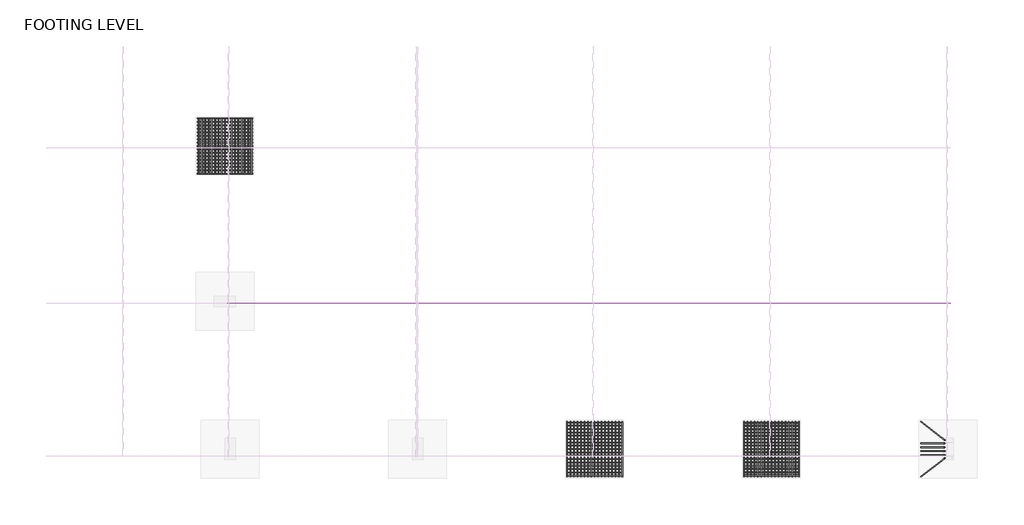
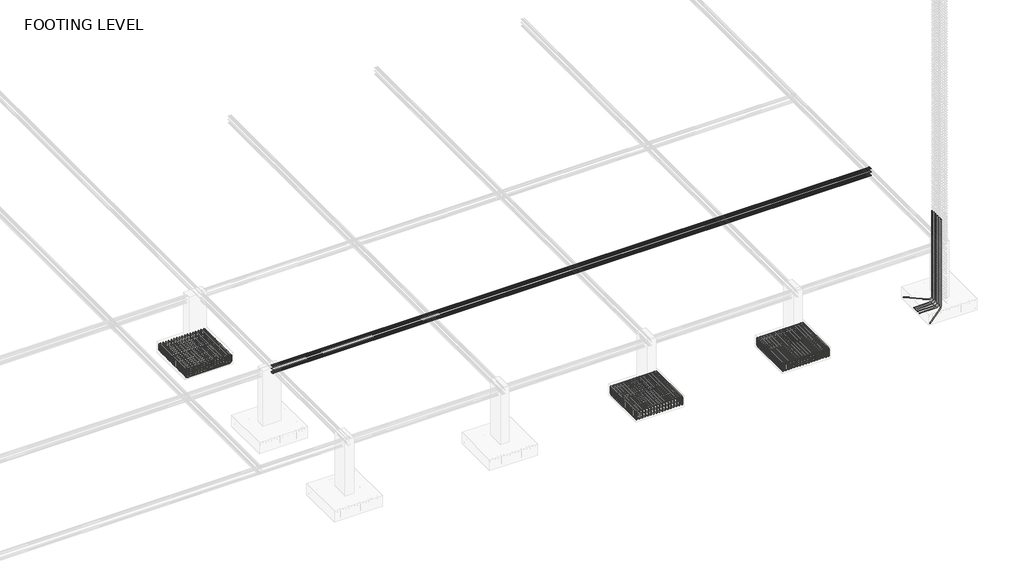
# One storey, part 6 of 19: 16 reinforcing bars.
"""IFC4 building model written with IfcOpenShell, lengths in millimetres."""

from ifc_helpers import new_model, si_unit, point, frame, origin, place, context, project, spatial, polyline, circle_curve, trimmed, segment, composite_curve, source, transform, mapped, element, save
from ifc_brep_helpers import swept_disk

model = new_model("IFC4")

# Units and contexts
model_context = context("Model", 3, world=origin())
ifc_project = project(units=[si_unit("LENGTHUNIT", "METRE", prefix="MILLI")], contexts=[model_context])

# Site, building, storey
site = spatial("IfcSite", under=ifc_project)
building = spatial("IfcBuilding", under=site)
storey = spatial("IfcBuildingStorey", under=building, Name="FOOTING LEVEL", Elevation=-3048.0)

# Reinforcing bars
placement = place(None, origin())
element("IfcReinforcingBar", 1, at=placement, inside=storey, context=model_context, shape_type="SolidModel", body=[
    swept_disk(composite_curve([segment(polyline([(32151.2177574, -27441.3062866, 1300.0821641), (32151.2177574, -27441.3062866, -3426.35)]), True, "CONTINUOUS"), segment(trimmed(circle_curve(frame((32030.1399051, -27346.7099009, -3426.35), z_axis=(0.6156614753255063, 0.7880107536068408, 0.0), x_axis=(121.07785230000081, -94.59638569999879, 0.0)), 153.65), [point((32151.2177574, -27441.3062866, -3426.35))], [point((32030.1399051, -27346.7099009, -3580.0))], True, "CARTESIAN"), True, "CONTINUOUS"), segment(polyline([(32030.1399051, -27346.7099009, -3580.0), (31124.1613605, -26638.881886, -3580.0)]), True, "CONTINUOUS")], self_intersect=False), 16.15),
])
element("IfcReinforcingBar", 2, at=placement, inside=storey, context=model_context, shape_type="SolidModel", body=[
    swept_disk(composite_curve([segment(polyline([(32151.8797141, -28220.6474683, 1296.5097943), (32151.8797141, -28220.6474683, -3426.35)]), True, "CONTINUOUS"), segment(trimmed(circle_curve(frame((32030.8018618, -28315.243854, -3426.35), z_axis=(-0.6156614753255063, 0.7880107536068408, 0.0), x_axis=(121.07785230000081, 94.59638569999879, 0.0)), 153.65), [point((32151.8797141, -28220.6474683, -3426.35))], [point((32030.8018618, -28315.243854, -3580.0))], True, "CARTESIAN"), True, "CONTINUOUS"), segment(polyline([(32030.8018618, -28315.243854, -3580.0), (31127.9113605, -29020.6592249, -3580.0)]), True, "CONTINUOUS")], self_intersect=False), 16.15),
])
reinforcing_bar_shape = source(origin(), model_context, "Body", "SolidModel", [
    swept_disk(composite_curve([segment(polyline([(32149.6087563, -28081.7876394, 1313.4672881), (32149.6087563, -28081.7876394, -3426.35)]), True, "CONTINUOUS"), segment(trimmed(circle_curve(frame((31995.9587563, -28081.7876394, -3426.35), z_axis=(0.0, 1.0, 0.0), x_axis=(153.65000000000146, 0.0, 0.0)), 153.65), [point((32149.6087563, -28081.7876394, -3426.35))], [point((31995.9587563, -28081.7876394, -3580.0))], True, "CARTESIAN"), True, "CONTINUOUS"), segment(polyline([(31995.9587563, -28081.7876394, -3580.0), (31112.5587563, -28081.7876394, -3580.0)]), True, "CONTINUOUS")], self_intersect=False), 16.15),
])
element("IfcReinforcingBar", 3, at=placement, inside=storey, context=model_context, shape_type="MappedRepresentation", body=[
    mapped(reinforcing_bar_shape, transform((0.0, 0.0, 0.0), x_axis=(1.0, 0.0, 0.0), y_axis=(0.0, 1.0, 0.0), z_axis=(0.0, 0.0, 1.0))),
    mapped(reinforcing_bar_shape, transform((0.0, 165.6818922, 0.0), x_axis=(1.0, 0.0, 0.0), y_axis=(0.0, 1.0, 0.0), z_axis=(0.0, 0.0, 1.0))),
    mapped(reinforcing_bar_shape, transform((0.0, 331.3637844, 0.0), x_axis=(1.0, 0.0, 0.0), y_axis=(0.0, 1.0, 0.0), z_axis=(0.0, 0.0, 1.0))),
    mapped(reinforcing_bar_shape, transform((0.0, 497.0456766, 0.0), x_axis=(1.0, 0.0, 0.0), y_axis=(0.0, 1.0, 0.0), z_axis=(0.0, 0.0, 1.0))),
])
reinforcing_bar_2_shape = source(origin(), model_context, "Body", "SolidModel", [
    swept_disk(composite_curve([segment(polyline([(25879.8587563, -28952.7516566, -3148.0), (25879.8587563, -28952.7516566, -3470.1)]), True, "CONTINUOUS"), segment(trimmed(circle_curve(frame((25789.6587563, -28952.7516566, -3470.1), z_axis=(0.0, 1.0, 0.0), x_axis=(90.20000000000073, 0.0, 0.0)), 90.2), [point((25879.8587563, -28952.7516566, -3470.1))], [point((25789.6587563, -28952.7516566, -3560.3))], True, "CARTESIAN"), True, "CONTINUOUS"), segment(polyline([(25789.6587563, -28952.7516566, -3560.3), (23595.4587563, -28952.7516566, -3560.3)]), True, "CONTINUOUS"), segment(trimmed(circle_curve(frame((23595.4587563, -28952.7516566, -3470.1), z_axis=(0.0, 1.0, 0.0), x_axis=(0.0, 0.0, -90.20000000000027)), 90.2), [point((23595.4587563, -28952.7516566, -3560.3))], [point((23505.2587563, -28952.7516566, -3470.1))], True, "CARTESIAN"), True, "CONTINUOUS"), segment(polyline([(23505.2587563, -28952.7516566, -3470.1), (23505.2587563, -28952.7516566, -3148.0)]), True, "CONTINUOUS")], self_intersect=False), 12.7),
])
element("IfcReinforcingBar", 4, at=placement, inside=storey, context=model_context, shape_type="MappedRepresentation", body=[
    mapped(reinforcing_bar_2_shape, transform((0.0, 0.0, 0.0), x_axis=(1.0, 0.0, 0.0), y_axis=(0.0, 1.0, 0.0), z_axis=(0.0, 0.0, 1.0))),
    mapped(reinforcing_bar_2_shape, transform((0.0, 140.8090411, 0.0), x_axis=(1.0, 0.0, 0.0), y_axis=(0.0, 1.0, 0.0), z_axis=(0.0, 0.0, 1.0))),
    mapped(reinforcing_bar_2_shape, transform((0.0, 281.6180821, 0.0), x_axis=(1.0, 0.0, 0.0), y_axis=(0.0, 1.0, 0.0), z_axis=(0.0, 0.0, 1.0))),
    mapped(reinforcing_bar_2_shape, transform((0.0, 422.4271232, 0.0), x_axis=(1.0, 0.0, 0.0), y_axis=(0.0, 1.0, 0.0), z_axis=(0.0, 0.0, 1.0))),
    mapped(reinforcing_bar_2_shape, transform((0.0, 563.2361643, 0.0), x_axis=(1.0, 0.0, 0.0), y_axis=(0.0, 1.0, 0.0), z_axis=(0.0, 0.0, 1.0))),
    mapped(reinforcing_bar_2_shape, transform((0.0, 704.0452054, 0.0), x_axis=(1.0, 0.0, 0.0), y_axis=(0.0, 1.0, 0.0), z_axis=(0.0, 0.0, 1.0))),
    mapped(reinforcing_bar_2_shape, transform((0.0, 844.8542464, 0.0), x_axis=(1.0, 0.0, 0.0), y_axis=(0.0, 1.0, 0.0), z_axis=(0.0, 0.0, 1.0))),
    mapped(reinforcing_bar_2_shape, transform((0.0, 985.6632875, 0.0), x_axis=(1.0, 0.0, 0.0), y_axis=(0.0, 1.0, 0.0), z_axis=(0.0, 0.0, 1.0))),
    mapped(reinforcing_bar_2_shape, transform((0.0, 1126.4723286, 0.0), x_axis=(1.0, 0.0, 0.0), y_axis=(0.0, 1.0, 0.0), z_axis=(0.0, 0.0, 1.0))),
    mapped(reinforcing_bar_2_shape, transform((0.0, 1267.2813697, 0.0), x_axis=(1.0, 0.0, 0.0), y_axis=(0.0, 1.0, 0.0), z_axis=(0.0, 0.0, 1.0))),
    mapped(reinforcing_bar_2_shape, transform((0.0, 1408.0904107, 0.0), x_axis=(1.0, 0.0, 0.0), y_axis=(0.0, 1.0, 0.0), z_axis=(0.0, 0.0, 1.0))),
    mapped(reinforcing_bar_2_shape, transform((0.0, 1548.8994518, 0.0), x_axis=(1.0, 0.0, 0.0), y_axis=(0.0, 1.0, 0.0), z_axis=(0.0, 0.0, 1.0))),
    mapped(reinforcing_bar_2_shape, transform((0.0, 1689.7084929, 0.0), x_axis=(1.0, 0.0, 0.0), y_axis=(0.0, 1.0, 0.0), z_axis=(0.0, 0.0, 1.0))),
    mapped(reinforcing_bar_2_shape, transform((0.0, 1830.517534, 0.0), x_axis=(1.0, 0.0, 0.0), y_axis=(0.0, 1.0, 0.0), z_axis=(0.0, 0.0, 1.0))),
    mapped(reinforcing_bar_2_shape, transform((0.0, 1971.326575, 0.0), x_axis=(1.0, 0.0, 0.0), y_axis=(0.0, 1.0, 0.0), z_axis=(0.0, 0.0, 1.0))),
    mapped(reinforcing_bar_2_shape, transform((0.0, 2112.1356161, 0.0), x_axis=(1.0, 0.0, 0.0), y_axis=(0.0, 1.0, 0.0), z_axis=(0.0, 0.0, 1.0))),
    mapped(reinforcing_bar_2_shape, transform((0.0, 2252.9446572, 0.0), x_axis=(1.0, 0.0, 0.0), y_axis=(0.0, 1.0, 0.0), z_axis=(0.0, 0.0, 1.0))),
])
reinforcing_bar_3_shape = source(origin(), model_context, "Body", "SolidModel", [
    swept_disk(composite_curve([segment(polyline([(25879.8587563, -26677.3596072, -3548.0), (25879.8587563, -26677.3596072, -3225.9)]), True, "CONTINUOUS"), segment(trimmed(circle_curve(frame((25789.6587563, -26677.3596072, -3225.9), z_axis=(0.0, -1.0, 0.0), x_axis=(90.20000000000073, 0.0, 0.0)), 90.2), [point((25879.8587563, -26677.3596072, -3225.9))], [point((25789.6587563, -26677.3596072, -3135.7))], True, "CARTESIAN"), True, "CONTINUOUS"), segment(polyline([(25789.6587563, -26677.3596072, -3135.7), (23595.4587563, -26677.3596072, -3135.7)]), True, "CONTINUOUS"), segment(trimmed(circle_curve(frame((23595.4587563, -26677.3596072, -3225.9), z_axis=(0.0, -1.0, 0.0), x_axis=(0.0, 0.0, 90.20000000000027)), 90.2), [point((23595.4587563, -26677.3596072, -3135.7))], [point((23505.2587563, -26677.3596072, -3225.9))], True, "CARTESIAN"), True, "CONTINUOUS"), segment(polyline([(23505.2587563, -26677.3596072, -3225.9), (23505.2587563, -26677.3596072, -3548.0)]), True, "CONTINUOUS")], self_intersect=False), 12.7),
])
element("IfcReinforcingBar", 5, at=placement, inside=storey, context=model_context, shape_type="MappedRepresentation", body=[
    mapped(reinforcing_bar_3_shape, transform((0.0, 0.0, 0.0), x_axis=(1.0, 0.0, 0.0), y_axis=(0.0, 1.0, 0.0), z_axis=(0.0, 0.0, 1.0))),
    mapped(reinforcing_bar_3_shape, transform((0.0, -143.8496077, 0.0), x_axis=(1.0, 0.0, 0.0), y_axis=(0.0, 1.0, 0.0), z_axis=(0.0, 0.0, 1.0))),
    mapped(reinforcing_bar_3_shape, transform((0.0, -287.6992155, 0.0), x_axis=(1.0, 0.0, 0.0), y_axis=(0.0, 1.0, 0.0), z_axis=(0.0, 0.0, 1.0))),
    mapped(reinforcing_bar_3_shape, transform((0.0, -431.5488232, 0.0), x_axis=(1.0, 0.0, 0.0), y_axis=(0.0, 1.0, 0.0), z_axis=(0.0, 0.0, 1.0))),
    mapped(reinforcing_bar_3_shape, transform((0.0, -575.398431, 0.0), x_axis=(1.0, 0.0, 0.0), y_axis=(0.0, 1.0, 0.0), z_axis=(0.0, 0.0, 1.0))),
    mapped(reinforcing_bar_3_shape, transform((0.0, -719.2480387, 0.0), x_axis=(1.0, 0.0, 0.0), y_axis=(0.0, 1.0, 0.0), z_axis=(0.0, 0.0, 1.0))),
    mapped(reinforcing_bar_3_shape, transform((0.0, -863.0976465, 0.0), x_axis=(1.0, 0.0, 0.0), y_axis=(0.0, 1.0, 0.0), z_axis=(0.0, 0.0, 1.0))),
    mapped(reinforcing_bar_3_shape, transform((0.0, -1006.9472542, 0.0), x_axis=(1.0, 0.0, 0.0), y_axis=(0.0, 1.0, 0.0), z_axis=(0.0, 0.0, 1.0))),
    mapped(reinforcing_bar_3_shape, transform((0.0, -1150.796862, 0.0), x_axis=(1.0, 0.0, 0.0), y_axis=(0.0, 1.0, 0.0), z_axis=(0.0, 0.0, 1.0))),
    mapped(reinforcing_bar_3_shape, transform((0.0, -1294.6464697, 0.0), x_axis=(1.0, 0.0, 0.0), y_axis=(0.0, 1.0, 0.0), z_axis=(0.0, 0.0, 1.0))),
    mapped(reinforcing_bar_3_shape, transform((0.0, -1438.4960775, 0.0), x_axis=(1.0, 0.0, 0.0), y_axis=(0.0, 1.0, 0.0), z_axis=(0.0, 0.0, 1.0))),
    mapped(reinforcing_bar_3_shape, transform((0.0, -1582.3456852, 0.0), x_axis=(1.0, 0.0, 0.0), y_axis=(0.0, 1.0, 0.0), z_axis=(0.0, 0.0, 1.0))),
    mapped(reinforcing_bar_3_shape, transform((0.0, -1726.195293, 0.0), x_axis=(1.0, 0.0, 0.0), y_axis=(0.0, 1.0, 0.0), z_axis=(0.0, 0.0, 1.0))),
    mapped(reinforcing_bar_3_shape, transform((0.0, -1870.0449007, 0.0), x_axis=(1.0, 0.0, 0.0), y_axis=(0.0, 1.0, 0.0), z_axis=(0.0, 0.0, 1.0))),
    mapped(reinforcing_bar_3_shape, transform((0.0, -2013.8945085, 0.0), x_axis=(1.0, 0.0, 0.0), y_axis=(0.0, 1.0, 0.0), z_axis=(0.0, 0.0, 1.0))),
    mapped(reinforcing_bar_3_shape, transform((0.0, -2157.7441162, 0.0), x_axis=(1.0, 0.0, 0.0), y_axis=(0.0, 1.0, 0.0), z_axis=(0.0, 0.0, 1.0))),
    mapped(reinforcing_bar_3_shape, transform((0.0, -2301.5937239, 0.0), x_axis=(1.0, 0.0, 0.0), y_axis=(0.0, 1.0, 0.0), z_axis=(0.0, 0.0, 1.0))),
])
reinforcing_bar_4_shape = source(origin(), model_context, "Body", "SolidModel", [
    swept_disk(composite_curve([segment(polyline([(23505.2587563, -29018.3205555, -3173.0), (23505.2587563, -29018.3205555, -3495.1)]), True, "CONTINUOUS"), segment(trimmed(circle_curve(frame((23505.2587563, -28928.1205555, -3495.1), z_axis=(1.0, 0.0, 0.0), x_axis=(0.0, -90.19999999999709, 0.0)), 90.2), [point((23505.2587563, -29018.3205555, -3495.1))], [point((23505.2587563, -28928.1205555, -3585.3))], True, "CARTESIAN"), True, "CONTINUOUS"), segment(polyline([(23505.2587563, -28928.1205555, -3585.3), (23505.2587563, -26733.9205555, -3585.3)]), True, "CONTINUOUS"), segment(trimmed(circle_curve(frame((23505.2587563, -26733.9205555, -3495.1), z_axis=(1.0, 0.0, 0.0), x_axis=(0.0, 0.0, -90.20000000000027)), 90.2), [point((23505.2587563, -26733.9205555, -3585.3))], [point((23505.2587563, -26643.7205555, -3495.1))], True, "CARTESIAN"), True, "CONTINUOUS"), segment(polyline([(23505.2587563, -26643.7205555, -3495.1), (23505.2587563, -26643.7205555, -3173.0)]), True, "CONTINUOUS")], self_intersect=False), 12.7),
])
element("IfcReinforcingBar", 6, at=placement, inside=storey, context=model_context, shape_type="MappedRepresentation", body=[
    mapped(reinforcing_bar_4_shape, transform((0.0, 0.0, 0.0), x_axis=(1.0, 0.0, 0.0), y_axis=(0.0, 1.0, 0.0), z_axis=(0.0, 0.0, 1.0))),
    mapped(reinforcing_bar_4_shape, transform((148.4125, 0.0, 0.0), x_axis=(1.0, 0.0, 0.0), y_axis=(0.0, 1.0, 0.0), z_axis=(0.0, 0.0, 1.0))),
    mapped(reinforcing_bar_4_shape, transform((296.825, 0.0, 0.0), x_axis=(1.0, 0.0, 0.0), y_axis=(0.0, 1.0, 0.0), z_axis=(0.0, 0.0, 1.0))),
    mapped(reinforcing_bar_4_shape, transform((445.2375, 0.0, 0.0), x_axis=(1.0, 0.0, 0.0), y_axis=(0.0, 1.0, 0.0), z_axis=(0.0, 0.0, 1.0))),
    mapped(reinforcing_bar_4_shape, transform((593.65, 0.0, 0.0), x_axis=(1.0, 0.0, 0.0), y_axis=(0.0, 1.0, 0.0), z_axis=(0.0, 0.0, 1.0))),
    mapped(reinforcing_bar_4_shape, transform((742.0625, 0.0, 0.0), x_axis=(1.0, 0.0, 0.0), y_axis=(0.0, 1.0, 0.0), z_axis=(0.0, 0.0, 1.0))),
    mapped(reinforcing_bar_4_shape, transform((890.475, 0.0, 0.0), x_axis=(1.0, 0.0, 0.0), y_axis=(0.0, 1.0, 0.0), z_axis=(0.0, 0.0, 1.0))),
    mapped(reinforcing_bar_4_shape, transform((1038.8875, 0.0, 0.0), x_axis=(1.0, 0.0, 0.0), y_axis=(0.0, 1.0, 0.0), z_axis=(0.0, 0.0, 1.0))),
    mapped(reinforcing_bar_4_shape, transform((1187.3, 0.0, 0.0), x_axis=(1.0, 0.0, 0.0), y_axis=(0.0, 1.0, 0.0), z_axis=(0.0, 0.0, 1.0))),
    mapped(reinforcing_bar_4_shape, transform((1335.7125, 0.0, 0.0), x_axis=(1.0, 0.0, 0.0), y_axis=(0.0, 1.0, 0.0), z_axis=(0.0, 0.0, 1.0))),
    mapped(reinforcing_bar_4_shape, transform((1484.125, 0.0, 0.0), x_axis=(1.0, 0.0, 0.0), y_axis=(0.0, 1.0, 0.0), z_axis=(0.0, 0.0, 1.0))),
    mapped(reinforcing_bar_4_shape, transform((1632.5375, 0.0, 0.0), x_axis=(1.0, 0.0, 0.0), y_axis=(0.0, 1.0, 0.0), z_axis=(0.0, 0.0, 1.0))),
    mapped(reinforcing_bar_4_shape, transform((1780.95, 0.0, 0.0), x_axis=(1.0, 0.0, 0.0), y_axis=(0.0, 1.0, 0.0), z_axis=(0.0, 0.0, 1.0))),
    mapped(reinforcing_bar_4_shape, transform((1929.3625, 0.0, 0.0), x_axis=(1.0, 0.0, 0.0), y_axis=(0.0, 1.0, 0.0), z_axis=(0.0, 0.0, 1.0))),
    mapped(reinforcing_bar_4_shape, transform((2077.775, 0.0, 0.0), x_axis=(1.0, 0.0, 0.0), y_axis=(0.0, 1.0, 0.0), z_axis=(0.0, 0.0, 1.0))),
    mapped(reinforcing_bar_4_shape, transform((2226.1875, 0.0, 0.0), x_axis=(1.0, 0.0, 0.0), y_axis=(0.0, 1.0, 0.0), z_axis=(0.0, 0.0, 1.0))),
    mapped(reinforcing_bar_4_shape, transform((2374.6, 0.0, 0.0), x_axis=(1.0, 0.0, 0.0), y_axis=(0.0, 1.0, 0.0), z_axis=(0.0, 0.0, 1.0))),
])
reinforcing_bar_5_shape = source(origin(), model_context, "Body", "SolidModel", [
    swept_disk(composite_curve([segment(polyline([(23505.2587563, -26643.7205555, -3523.0), (23505.2587563, -26643.7205555, -3200.9)]), True, "CONTINUOUS"), segment(trimmed(circle_curve(frame((23505.2587563, -26733.9205555, -3200.9), z_axis=(1.0, 0.0, 0.0), x_axis=(0.0, 90.20000000000073, 0.0)), 90.2), [point((23505.2587563, -26643.7205555, -3200.9))], [point((23505.2587563, -26733.9205555, -3110.7))], True, "CARTESIAN"), True, "CONTINUOUS"), segment(polyline([(23505.2587563, -26733.9205555, -3110.7), (23505.2587563, -28928.1205555, -3110.7)]), True, "CONTINUOUS"), segment(trimmed(circle_curve(frame((23505.2587563, -28928.1205555, -3200.9), z_axis=(1.0, 0.0, 0.0), x_axis=(0.0, 0.0, 90.20000000000027)), 90.2), [point((23505.2587563, -28928.1205555, -3110.7))], [point((23505.2587563, -29018.3205555, -3200.9))], True, "CARTESIAN"), True, "CONTINUOUS"), segment(polyline([(23505.2587563, -29018.3205555, -3200.9), (23505.2587563, -29018.3205555, -3523.0)]), True, "CONTINUOUS")], self_intersect=False), 12.7),
])
element("IfcReinforcingBar", 7, at=placement, inside=storey, context=model_context, shape_type="MappedRepresentation", body=[
    mapped(reinforcing_bar_5_shape, transform((0.0, 0.0, 0.0), x_axis=(1.0, 0.0, 0.0), y_axis=(0.0, 1.0, 0.0), z_axis=(0.0, 0.0, 1.0))),
    mapped(reinforcing_bar_5_shape, transform((148.4125, 0.0, 0.0), x_axis=(1.0, 0.0, 0.0), y_axis=(0.0, 1.0, 0.0), z_axis=(0.0, 0.0, 1.0))),
    mapped(reinforcing_bar_5_shape, transform((296.825, 0.0, 0.0), x_axis=(1.0, 0.0, 0.0), y_axis=(0.0, 1.0, 0.0), z_axis=(0.0, 0.0, 1.0))),
    mapped(reinforcing_bar_5_shape, transform((445.2375, 0.0, 0.0), x_axis=(1.0, 0.0, 0.0), y_axis=(0.0, 1.0, 0.0), z_axis=(0.0, 0.0, 1.0))),
    mapped(reinforcing_bar_5_shape, transform((593.65, 0.0, 0.0), x_axis=(1.0, 0.0, 0.0), y_axis=(0.0, 1.0, 0.0), z_axis=(0.0, 0.0, 1.0))),
    mapped(reinforcing_bar_5_shape, transform((742.0625, 0.0, 0.0), x_axis=(1.0, 0.0, 0.0), y_axis=(0.0, 1.0, 0.0), z_axis=(0.0, 0.0, 1.0))),
    mapped(reinforcing_bar_5_shape, transform((890.475, 0.0, 0.0), x_axis=(1.0, 0.0, 0.0), y_axis=(0.0, 1.0, 0.0), z_axis=(0.0, 0.0, 1.0))),
    mapped(reinforcing_bar_5_shape, transform((1038.8875, 0.0, 0.0), x_axis=(1.0, 0.0, 0.0), y_axis=(0.0, 1.0, 0.0), z_axis=(0.0, 0.0, 1.0))),
    mapped(reinforcing_bar_5_shape, transform((1187.3, 0.0, 0.0), x_axis=(1.0, 0.0, 0.0), y_axis=(0.0, 1.0, 0.0), z_axis=(0.0, 0.0, 1.0))),
    mapped(reinforcing_bar_5_shape, transform((1335.7125, 0.0, 0.0), x_axis=(1.0, 0.0, 0.0), y_axis=(0.0, 1.0, 0.0), z_axis=(0.0, 0.0, 1.0))),
    mapped(reinforcing_bar_5_shape, transform((1484.125, 0.0, 0.0), x_axis=(1.0, 0.0, 0.0), y_axis=(0.0, 1.0, 0.0), z_axis=(0.0, 0.0, 1.0))),
    mapped(reinforcing_bar_5_shape, transform((1632.5375, 0.0, 0.0), x_axis=(1.0, 0.0, 0.0), y_axis=(0.0, 1.0, 0.0), z_axis=(0.0, 0.0, 1.0))),
    mapped(reinforcing_bar_5_shape, transform((1780.95, 0.0, 0.0), x_axis=(1.0, 0.0, 0.0), y_axis=(0.0, 1.0, 0.0), z_axis=(0.0, 0.0, 1.0))),
    mapped(reinforcing_bar_5_shape, transform((1929.3625, 0.0, 0.0), x_axis=(1.0, 0.0, 0.0), y_axis=(0.0, 1.0, 0.0), z_axis=(0.0, 0.0, 1.0))),
    mapped(reinforcing_bar_5_shape, transform((2077.775, 0.0, 0.0), x_axis=(1.0, 0.0, 0.0), y_axis=(0.0, 1.0, 0.0), z_axis=(0.0, 0.0, 1.0))),
    mapped(reinforcing_bar_5_shape, transform((2226.1875, 0.0, 0.0), x_axis=(1.0, 0.0, 0.0), y_axis=(0.0, 1.0, 0.0), z_axis=(0.0, 0.0, 1.0))),
    mapped(reinforcing_bar_5_shape, transform((2374.6, 0.0, 0.0), x_axis=(1.0, 0.0, 0.0), y_axis=(0.0, 1.0, 0.0), z_axis=(0.0, 0.0, 1.0))),
])
reinforcing_bar_6_shape = source(origin(), model_context, "Body", "SolidModel", [
    swept_disk(composite_curve([segment(polyline([(18259.8587563, -26677.3596072, -3548.0), (18259.8587563, -26677.3596072, -3225.9)]), True, "CONTINUOUS"), segment(trimmed(circle_curve(frame((18169.6587563, -26677.3596072, -3225.9), z_axis=(0.0, -1.0, 0.0), x_axis=(90.20000000000073, 0.0, 0.0)), 90.2), [point((18259.8587563, -26677.3596072, -3225.9))], [point((18169.6587563, -26677.3596072, -3135.7))], True, "CARTESIAN"), True, "CONTINUOUS"), segment(polyline([(18169.6587563, -26677.3596072, -3135.7), (15975.4587563, -26677.3596072, -3135.7)]), True, "CONTINUOUS"), segment(trimmed(circle_curve(frame((15975.4587563, -26677.3596072, -3225.9), z_axis=(0.0, -1.0, 0.0), x_axis=(0.0, 0.0, 90.20000000000027)), 90.2), [point((15975.4587563, -26677.3596072, -3135.7))], [point((15885.2587563, -26677.3596072, -3225.9))], True, "CARTESIAN"), True, "CONTINUOUS"), segment(polyline([(15885.2587563, -26677.3596072, -3225.9), (15885.2587563, -26677.3596072, -3548.0)]), True, "CONTINUOUS")], self_intersect=False), 12.7),
])
element("IfcReinforcingBar", 8, at=placement, inside=storey, context=model_context, shape_type="MappedRepresentation", body=[
    mapped(reinforcing_bar_6_shape, transform((0.0, 0.0, 0.0), x_axis=(1.0, 0.0, 0.0), y_axis=(0.0, 1.0, 0.0), z_axis=(0.0, 0.0, 1.0))),
    mapped(reinforcing_bar_6_shape, transform((0.0, -143.8496077, 0.0), x_axis=(1.0, 0.0, 0.0), y_axis=(0.0, 1.0, 0.0), z_axis=(0.0, 0.0, 1.0))),
    mapped(reinforcing_bar_6_shape, transform((0.0, -287.6992155, 0.0), x_axis=(1.0, 0.0, 0.0), y_axis=(0.0, 1.0, 0.0), z_axis=(0.0, 0.0, 1.0))),
    mapped(reinforcing_bar_6_shape, transform((0.0, -431.5488232, 0.0), x_axis=(1.0, 0.0, 0.0), y_axis=(0.0, 1.0, 0.0), z_axis=(0.0, 0.0, 1.0))),
    mapped(reinforcing_bar_6_shape, transform((0.0, -575.398431, 0.0), x_axis=(1.0, 0.0, 0.0), y_axis=(0.0, 1.0, 0.0), z_axis=(0.0, 0.0, 1.0))),
    mapped(reinforcing_bar_6_shape, transform((0.0, -719.2480387, 0.0), x_axis=(1.0, 0.0, 0.0), y_axis=(0.0, 1.0, 0.0), z_axis=(0.0, 0.0, 1.0))),
    mapped(reinforcing_bar_6_shape, transform((0.0, -863.0976465, 0.0), x_axis=(1.0, 0.0, 0.0), y_axis=(0.0, 1.0, 0.0), z_axis=(0.0, 0.0, 1.0))),
    mapped(reinforcing_bar_6_shape, transform((0.0, -1006.9472542, 0.0), x_axis=(1.0, 0.0, 0.0), y_axis=(0.0, 1.0, 0.0), z_axis=(0.0, 0.0, 1.0))),
    mapped(reinforcing_bar_6_shape, transform((0.0, -1150.796862, 0.0), x_axis=(1.0, 0.0, 0.0), y_axis=(0.0, 1.0, 0.0), z_axis=(0.0, 0.0, 1.0))),
    mapped(reinforcing_bar_6_shape, transform((0.0, -1294.6464697, 0.0), x_axis=(1.0, 0.0, 0.0), y_axis=(0.0, 1.0, 0.0), z_axis=(0.0, 0.0, 1.0))),
    mapped(reinforcing_bar_6_shape, transform((0.0, -1438.4960775, 0.0), x_axis=(1.0, 0.0, 0.0), y_axis=(0.0, 1.0, 0.0), z_axis=(0.0, 0.0, 1.0))),
    mapped(reinforcing_bar_6_shape, transform((0.0, -1582.3456852, 0.0), x_axis=(1.0, 0.0, 0.0), y_axis=(0.0, 1.0, 0.0), z_axis=(0.0, 0.0, 1.0))),
    mapped(reinforcing_bar_6_shape, transform((0.0, -1726.195293, 0.0), x_axis=(1.0, 0.0, 0.0), y_axis=(0.0, 1.0, 0.0), z_axis=(0.0, 0.0, 1.0))),
    mapped(reinforcing_bar_6_shape, transform((0.0, -1870.0449007, 0.0), x_axis=(1.0, 0.0, 0.0), y_axis=(0.0, 1.0, 0.0), z_axis=(0.0, 0.0, 1.0))),
    mapped(reinforcing_bar_6_shape, transform((0.0, -2013.8945085, 0.0), x_axis=(1.0, 0.0, 0.0), y_axis=(0.0, 1.0, 0.0), z_axis=(0.0, 0.0, 1.0))),
    mapped(reinforcing_bar_6_shape, transform((0.0, -2157.7441162, 0.0), x_axis=(1.0, 0.0, 0.0), y_axis=(0.0, 1.0, 0.0), z_axis=(0.0, 0.0, 1.0))),
    mapped(reinforcing_bar_6_shape, transform((0.0, -2301.5937239, 0.0), x_axis=(1.0, 0.0, 0.0), y_axis=(0.0, 1.0, 0.0), z_axis=(0.0, 0.0, 1.0))),
])
reinforcing_bar_7_shape = source(origin(), model_context, "Body", "SolidModel", [
    swept_disk(composite_curve([segment(polyline([(15885.2587563, -29018.3205555, -3173.0), (15885.2587563, -29018.3205555, -3495.1)]), True, "CONTINUOUS"), segment(trimmed(circle_curve(frame((15885.2587563, -28928.1205555, -3495.1), z_axis=(1.0, 0.0, 0.0), x_axis=(0.0, -90.19999999999709, 0.0)), 90.2), [point((15885.2587563, -29018.3205555, -3495.1))], [point((15885.2587563, -28928.1205555, -3585.3))], True, "CARTESIAN"), True, "CONTINUOUS"), segment(polyline([(15885.2587563, -28928.1205555, -3585.3), (15885.2587563, -26733.9205555, -3585.3)]), True, "CONTINUOUS"), segment(trimmed(circle_curve(frame((15885.2587563, -26733.9205555, -3495.1), z_axis=(1.0, 0.0, 0.0), x_axis=(0.0, 0.0, -90.20000000000027)), 90.2), [point((15885.2587563, -26733.9205555, -3585.3))], [point((15885.2587563, -26643.7205555, -3495.1))], True, "CARTESIAN"), True, "CONTINUOUS"), segment(polyline([(15885.2587563, -26643.7205555, -3495.1), (15885.2587563, -26643.7205555, -3173.0)]), True, "CONTINUOUS")], self_intersect=False), 12.7),
])
element("IfcReinforcingBar", 9, at=placement, inside=storey, context=model_context, shape_type="MappedRepresentation", body=[
    mapped(reinforcing_bar_7_shape, transform((0.0, 0.0, 0.0), x_axis=(1.0, 0.0, 0.0), y_axis=(0.0, 1.0, 0.0), z_axis=(0.0, 0.0, 1.0))),
    mapped(reinforcing_bar_7_shape, transform((148.4125, 0.0, 0.0), x_axis=(1.0, 0.0, 0.0), y_axis=(0.0, 1.0, 0.0), z_axis=(0.0, 0.0, 1.0))),
    mapped(reinforcing_bar_7_shape, transform((296.825, 0.0, 0.0), x_axis=(1.0, 0.0, 0.0), y_axis=(0.0, 1.0, 0.0), z_axis=(0.0, 0.0, 1.0))),
    mapped(reinforcing_bar_7_shape, transform((445.2375, 0.0, 0.0), x_axis=(1.0, 0.0, 0.0), y_axis=(0.0, 1.0, 0.0), z_axis=(0.0, 0.0, 1.0))),
    mapped(reinforcing_bar_7_shape, transform((593.65, 0.0, 0.0), x_axis=(1.0, 0.0, 0.0), y_axis=(0.0, 1.0, 0.0), z_axis=(0.0, 0.0, 1.0))),
    mapped(reinforcing_bar_7_shape, transform((742.0625, 0.0, 0.0), x_axis=(1.0, 0.0, 0.0), y_axis=(0.0, 1.0, 0.0), z_axis=(0.0, 0.0, 1.0))),
    mapped(reinforcing_bar_7_shape, transform((890.475, 0.0, 0.0), x_axis=(1.0, 0.0, 0.0), y_axis=(0.0, 1.0, 0.0), z_axis=(0.0, 0.0, 1.0))),
    mapped(reinforcing_bar_7_shape, transform((1038.8875, 0.0, 0.0), x_axis=(1.0, 0.0, 0.0), y_axis=(0.0, 1.0, 0.0), z_axis=(0.0, 0.0, 1.0))),
    mapped(reinforcing_bar_7_shape, transform((1187.3, 0.0, 0.0), x_axis=(1.0, 0.0, 0.0), y_axis=(0.0, 1.0, 0.0), z_axis=(0.0, 0.0, 1.0))),
    mapped(reinforcing_bar_7_shape, transform((1335.7125, 0.0, 0.0), x_axis=(1.0, 0.0, 0.0), y_axis=(0.0, 1.0, 0.0), z_axis=(0.0, 0.0, 1.0))),
    mapped(reinforcing_bar_7_shape, transform((1484.125, 0.0, 0.0), x_axis=(1.0, 0.0, 0.0), y_axis=(0.0, 1.0, 0.0), z_axis=(0.0, 0.0, 1.0))),
    mapped(reinforcing_bar_7_shape, transform((1632.5375, 0.0, 0.0), x_axis=(1.0, 0.0, 0.0), y_axis=(0.0, 1.0, 0.0), z_axis=(0.0, 0.0, 1.0))),
    mapped(reinforcing_bar_7_shape, transform((1780.95, 0.0, 0.0), x_axis=(1.0, 0.0, 0.0), y_axis=(0.0, 1.0, 0.0), z_axis=(0.0, 0.0, 1.0))),
    mapped(reinforcing_bar_7_shape, transform((1929.3625, 0.0, 0.0), x_axis=(1.0, 0.0, 0.0), y_axis=(0.0, 1.0, 0.0), z_axis=(0.0, 0.0, 1.0))),
    mapped(reinforcing_bar_7_shape, transform((2077.775, 0.0, 0.0), x_axis=(1.0, 0.0, 0.0), y_axis=(0.0, 1.0, 0.0), z_axis=(0.0, 0.0, 1.0))),
    mapped(reinforcing_bar_7_shape, transform((2226.1875, 0.0, 0.0), x_axis=(1.0, 0.0, 0.0), y_axis=(0.0, 1.0, 0.0), z_axis=(0.0, 0.0, 1.0))),
    mapped(reinforcing_bar_7_shape, transform((2374.6, 0.0, 0.0), x_axis=(1.0, 0.0, 0.0), y_axis=(0.0, 1.0, 0.0), z_axis=(0.0, 0.0, 1.0))),
])
reinforcing_bar_8_shape = source(origin(), model_context, "Body", "SolidModel", [
    swept_disk(composite_curve([segment(polyline([(15885.2587563, -26643.7205555, -3523.0), (15885.2587563, -26643.7205555, -3200.9)]), True, "CONTINUOUS"), segment(trimmed(circle_curve(frame((15885.2587563, -26733.9205555, -3200.9), z_axis=(1.0, 0.0, 0.0), x_axis=(0.0, 90.20000000000073, 0.0)), 90.2), [point((15885.2587563, -26643.7205555, -3200.9))], [point((15885.2587563, -26733.9205555, -3110.7))], True, "CARTESIAN"), True, "CONTINUOUS"), segment(polyline([(15885.2587563, -26733.9205555, -3110.7), (15885.2587563, -28928.1205555, -3110.7)]), True, "CONTINUOUS"), segment(trimmed(circle_curve(frame((15885.2587563, -28928.1205555, -3200.9), z_axis=(1.0, 0.0, 0.0), x_axis=(0.0, 0.0, 90.20000000000027)), 90.2), [point((15885.2587563, -28928.1205555, -3110.7))], [point((15885.2587563, -29018.3205555, -3200.9))], True, "CARTESIAN"), True, "CONTINUOUS"), segment(polyline([(15885.2587563, -29018.3205555, -3200.9), (15885.2587563, -29018.3205555, -3523.0)]), True, "CONTINUOUS")], self_intersect=False), 12.7),
])
element("IfcReinforcingBar", 10, at=placement, inside=storey, context=model_context, shape_type="MappedRepresentation", body=[
    mapped(reinforcing_bar_8_shape, transform((0.0, 0.0, 0.0), x_axis=(1.0, 0.0, 0.0), y_axis=(0.0, 1.0, 0.0), z_axis=(0.0, 0.0, 1.0))),
    mapped(reinforcing_bar_8_shape, transform((148.4125, 0.0, 0.0), x_axis=(1.0, 0.0, 0.0), y_axis=(0.0, 1.0, 0.0), z_axis=(0.0, 0.0, 1.0))),
    mapped(reinforcing_bar_8_shape, transform((296.825, 0.0, 0.0), x_axis=(1.0, 0.0, 0.0), y_axis=(0.0, 1.0, 0.0), z_axis=(0.0, 0.0, 1.0))),
    mapped(reinforcing_bar_8_shape, transform((445.2375, 0.0, 0.0), x_axis=(1.0, 0.0, 0.0), y_axis=(0.0, 1.0, 0.0), z_axis=(0.0, 0.0, 1.0))),
    mapped(reinforcing_bar_8_shape, transform((593.65, 0.0, 0.0), x_axis=(1.0, 0.0, 0.0), y_axis=(0.0, 1.0, 0.0), z_axis=(0.0, 0.0, 1.0))),
    mapped(reinforcing_bar_8_shape, transform((742.0625, 0.0, 0.0), x_axis=(1.0, 0.0, 0.0), y_axis=(0.0, 1.0, 0.0), z_axis=(0.0, 0.0, 1.0))),
    mapped(reinforcing_bar_8_shape, transform((890.475, 0.0, 0.0), x_axis=(1.0, 0.0, 0.0), y_axis=(0.0, 1.0, 0.0), z_axis=(0.0, 0.0, 1.0))),
    mapped(reinforcing_bar_8_shape, transform((1038.8875, 0.0, 0.0), x_axis=(1.0, 0.0, 0.0), y_axis=(0.0, 1.0, 0.0), z_axis=(0.0, 0.0, 1.0))),
    mapped(reinforcing_bar_8_shape, transform((1187.3, 0.0, 0.0), x_axis=(1.0, 0.0, 0.0), y_axis=(0.0, 1.0, 0.0), z_axis=(0.0, 0.0, 1.0))),
    mapped(reinforcing_bar_8_shape, transform((1335.7125, 0.0, 0.0), x_axis=(1.0, 0.0, 0.0), y_axis=(0.0, 1.0, 0.0), z_axis=(0.0, 0.0, 1.0))),
    mapped(reinforcing_bar_8_shape, transform((1484.125, 0.0, 0.0), x_axis=(1.0, 0.0, 0.0), y_axis=(0.0, 1.0, 0.0), z_axis=(0.0, 0.0, 1.0))),
    mapped(reinforcing_bar_8_shape, transform((1632.5375, 0.0, 0.0), x_axis=(1.0, 0.0, 0.0), y_axis=(0.0, 1.0, 0.0), z_axis=(0.0, 0.0, 1.0))),
    mapped(reinforcing_bar_8_shape, transform((1780.95, 0.0, 0.0), x_axis=(1.0, 0.0, 0.0), y_axis=(0.0, 1.0, 0.0), z_axis=(0.0, 0.0, 1.0))),
    mapped(reinforcing_bar_8_shape, transform((1929.3625, 0.0, 0.0), x_axis=(1.0, 0.0, 0.0), y_axis=(0.0, 1.0, 0.0), z_axis=(0.0, 0.0, 1.0))),
    mapped(reinforcing_bar_8_shape, transform((2077.775, 0.0, 0.0), x_axis=(1.0, 0.0, 0.0), y_axis=(0.0, 1.0, 0.0), z_axis=(0.0, 0.0, 1.0))),
    mapped(reinforcing_bar_8_shape, transform((2226.1875, 0.0, 0.0), x_axis=(1.0, 0.0, 0.0), y_axis=(0.0, 1.0, 0.0), z_axis=(0.0, 0.0, 1.0))),
    mapped(reinforcing_bar_8_shape, transform((2374.6, 0.0, 0.0), x_axis=(1.0, 0.0, 0.0), y_axis=(0.0, 1.0, 0.0), z_axis=(0.0, 0.0, 1.0))),
])
reinforcing_bar_9_shape = source(origin(), model_context, "Body", "SolidModel", [
    swept_disk(composite_curve([segment(polyline([(25.0276552, -15950.0205555, -3148.0), (25.0276552, -15950.0205555, -3470.1)]), True, "CONTINUOUS"), segment(trimmed(circle_curve(frame((25.0276552, -15859.8205555, -3470.1), z_axis=(1.0, 0.0, 0.0), x_axis=(0.0, -90.19999999999891, 0.0)), 90.2), [point((25.0276552, -15950.0205555, -3470.1))], [point((25.0276552, -15859.8205555, -3560.3))], True, "CARTESIAN"), True, "CONTINUOUS"), segment(polyline([(25.0276552, -15859.8205555, -3560.3), (25.0276552, -13665.6205555, -3560.3)]), True, "CONTINUOUS"), segment(trimmed(circle_curve(frame((25.0276552, -13665.6205555, -3470.1), z_axis=(1.0, 0.0, 0.0), x_axis=(0.0, 0.0, -90.20000000000027)), 90.2), [point((25.0276552, -13665.6205555, -3560.3))], [point((25.0276552, -13575.4205555, -3470.1))], True, "CARTESIAN"), True, "CONTINUOUS"), segment(polyline([(25.0276552, -13575.4205555, -3470.1), (25.0276552, -13575.4205555, -3148.0)]), True, "CONTINUOUS")], self_intersect=False), 12.7),
])
element("IfcReinforcingBar", 11, at=placement, inside=storey, context=model_context, shape_type="MappedRepresentation", body=[
    mapped(reinforcing_bar_9_shape, transform((0.0, 0.0, 0.0), x_axis=(1.0, 0.0, 0.0), y_axis=(0.0, 1.0, 0.0), z_axis=(0.0, 0.0, 1.0))),
    mapped(reinforcing_bar_9_shape, transform((140.8090411, 0.0, 0.0), x_axis=(1.0, 0.0, 0.0), y_axis=(0.0, 1.0, 0.0), z_axis=(0.0, 0.0, 1.0))),
    mapped(reinforcing_bar_9_shape, transform((281.6180821, 0.0, 0.0), x_axis=(1.0, 0.0, 0.0), y_axis=(0.0, 1.0, 0.0), z_axis=(0.0, 0.0, 1.0))),
    mapped(reinforcing_bar_9_shape, transform((422.4271232, 0.0, 0.0), x_axis=(1.0, 0.0, 0.0), y_axis=(0.0, 1.0, 0.0), z_axis=(0.0, 0.0, 1.0))),
    mapped(reinforcing_bar_9_shape, transform((563.2361643, 0.0, 0.0), x_axis=(1.0, 0.0, 0.0), y_axis=(0.0, 1.0, 0.0), z_axis=(0.0, 0.0, 1.0))),
    mapped(reinforcing_bar_9_shape, transform((704.0452054, 0.0, 0.0), x_axis=(1.0, 0.0, 0.0), y_axis=(0.0, 1.0, 0.0), z_axis=(0.0, 0.0, 1.0))),
    mapped(reinforcing_bar_9_shape, transform((844.8542464, 0.0, 0.0), x_axis=(1.0, 0.0, 0.0), y_axis=(0.0, 1.0, 0.0), z_axis=(0.0, 0.0, 1.0))),
    mapped(reinforcing_bar_9_shape, transform((985.6632875, 0.0, 0.0), x_axis=(1.0, 0.0, 0.0), y_axis=(0.0, 1.0, 0.0), z_axis=(0.0, 0.0, 1.0))),
    mapped(reinforcing_bar_9_shape, transform((1126.4723286, 0.0, 0.0), x_axis=(1.0, 0.0, 0.0), y_axis=(0.0, 1.0, 0.0), z_axis=(0.0, 0.0, 1.0))),
    mapped(reinforcing_bar_9_shape, transform((1267.2813697, 0.0, 0.0), x_axis=(1.0, 0.0, 0.0), y_axis=(0.0, 1.0, 0.0), z_axis=(0.0, 0.0, 1.0))),
    mapped(reinforcing_bar_9_shape, transform((1408.0904107, 0.0, 0.0), x_axis=(1.0, 0.0, 0.0), y_axis=(0.0, 1.0, 0.0), z_axis=(0.0, 0.0, 1.0))),
    mapped(reinforcing_bar_9_shape, transform((1548.8994518, 0.0, 0.0), x_axis=(1.0, 0.0, 0.0), y_axis=(0.0, 1.0, 0.0), z_axis=(0.0, 0.0, 1.0))),
    mapped(reinforcing_bar_9_shape, transform((1689.7084929, 0.0, 0.0), x_axis=(1.0, 0.0, 0.0), y_axis=(0.0, 1.0, 0.0), z_axis=(0.0, 0.0, 1.0))),
    mapped(reinforcing_bar_9_shape, transform((1830.517534, 0.0, 0.0), x_axis=(1.0, 0.0, 0.0), y_axis=(0.0, 1.0, 0.0), z_axis=(0.0, 0.0, 1.0))),
    mapped(reinforcing_bar_9_shape, transform((1971.326575, 0.0, 0.0), x_axis=(1.0, 0.0, 0.0), y_axis=(0.0, 1.0, 0.0), z_axis=(0.0, 0.0, 1.0))),
    mapped(reinforcing_bar_9_shape, transform((2112.1356161, 0.0, 0.0), x_axis=(1.0, 0.0, 0.0), y_axis=(0.0, 1.0, 0.0), z_axis=(0.0, 0.0, 1.0))),
    mapped(reinforcing_bar_9_shape, transform((2252.9446572, 0.0, 0.0), x_axis=(1.0, 0.0, 0.0), y_axis=(0.0, 1.0, 0.0), z_axis=(0.0, 0.0, 1.0))),
])
reinforcing_bar_10_shape = source(origin(), model_context, "Body", "SolidModel", [
    swept_disk(composite_curve([segment(polyline([(2300.4197045, -15950.0205555, -3548.0), (2300.4197045, -15950.0205555, -3225.9)]), True, "CONTINUOUS"), segment(trimmed(circle_curve(frame((2300.4197045, -15859.8205555, -3225.9), z_axis=(-1.0, 0.0, 0.0), x_axis=(0.0, -90.19999999999891, 0.0)), 90.2), [point((2300.4197045, -15950.0205555, -3225.9))], [point((2300.4197045, -15859.8205555, -3135.7))], True, "CARTESIAN"), True, "CONTINUOUS"), segment(polyline([(2300.4197045, -15859.8205555, -3135.7), (2300.4197045, -13665.6205555, -3135.7)]), True, "CONTINUOUS"), segment(trimmed(circle_curve(frame((2300.4197045, -13665.6205555, -3225.9), z_axis=(-1.0, 0.0, 0.0), x_axis=(0.0, 0.0, 90.20000000000027)), 90.2), [point((2300.4197045, -13665.6205555, -3135.7))], [point((2300.4197045, -13575.4205555, -3225.9))], True, "CARTESIAN"), True, "CONTINUOUS"), segment(polyline([(2300.4197045, -13575.4205555, -3225.9), (2300.4197045, -13575.4205555, -3548.0)]), True, "CONTINUOUS")], self_intersect=False), 12.7),
])
element("IfcReinforcingBar", 12, at=placement, inside=storey, context=model_context, shape_type="MappedRepresentation", body=[
    mapped(reinforcing_bar_10_shape, transform((0.0, 0.0, 0.0), x_axis=(1.0, 0.0, 0.0), y_axis=(0.0, 1.0, 0.0), z_axis=(0.0, 0.0, 1.0))),
    mapped(reinforcing_bar_10_shape, transform((-143.8496077, 0.0, 0.0), x_axis=(1.0, 0.0, 0.0), y_axis=(0.0, 1.0, 0.0), z_axis=(0.0, 0.0, 1.0))),
    mapped(reinforcing_bar_10_shape, transform((-287.6992155, 0.0, 0.0), x_axis=(1.0, 0.0, 0.0), y_axis=(0.0, 1.0, 0.0), z_axis=(0.0, 0.0, 1.0))),
    mapped(reinforcing_bar_10_shape, transform((-431.5488232, 0.0, 0.0), x_axis=(1.0, 0.0, 0.0), y_axis=(0.0, 1.0, 0.0), z_axis=(0.0, 0.0, 1.0))),
    mapped(reinforcing_bar_10_shape, transform((-575.398431, 0.0, 0.0), x_axis=(1.0, 0.0, 0.0), y_axis=(0.0, 1.0, 0.0), z_axis=(0.0, 0.0, 1.0))),
    mapped(reinforcing_bar_10_shape, transform((-719.2480387, 0.0, 0.0), x_axis=(1.0, 0.0, 0.0), y_axis=(0.0, 1.0, 0.0), z_axis=(0.0, 0.0, 1.0))),
    mapped(reinforcing_bar_10_shape, transform((-863.0976465, 0.0, 0.0), x_axis=(1.0, 0.0, 0.0), y_axis=(0.0, 1.0, 0.0), z_axis=(0.0, 0.0, 1.0))),
    mapped(reinforcing_bar_10_shape, transform((-1006.9472542, 0.0, 0.0), x_axis=(1.0, 0.0, 0.0), y_axis=(0.0, 1.0, 0.0), z_axis=(0.0, 0.0, 1.0))),
    mapped(reinforcing_bar_10_shape, transform((-1150.796862, 0.0, 0.0), x_axis=(1.0, 0.0, 0.0), y_axis=(0.0, 1.0, 0.0), z_axis=(0.0, 0.0, 1.0))),
    mapped(reinforcing_bar_10_shape, transform((-1294.6464697, 0.0, 0.0), x_axis=(1.0, 0.0, 0.0), y_axis=(0.0, 1.0, 0.0), z_axis=(0.0, 0.0, 1.0))),
    mapped(reinforcing_bar_10_shape, transform((-1438.4960775, 0.0, 0.0), x_axis=(1.0, 0.0, 0.0), y_axis=(0.0, 1.0, 0.0), z_axis=(0.0, 0.0, 1.0))),
    mapped(reinforcing_bar_10_shape, transform((-1582.3456852, 0.0, 0.0), x_axis=(1.0, 0.0, 0.0), y_axis=(0.0, 1.0, 0.0), z_axis=(0.0, 0.0, 1.0))),
    mapped(reinforcing_bar_10_shape, transform((-1726.195293, 0.0, 0.0), x_axis=(1.0, 0.0, 0.0), y_axis=(0.0, 1.0, 0.0), z_axis=(0.0, 0.0, 1.0))),
    mapped(reinforcing_bar_10_shape, transform((-1870.0449007, 0.0, 0.0), x_axis=(1.0, 0.0, 0.0), y_axis=(0.0, 1.0, 0.0), z_axis=(0.0, 0.0, 1.0))),
    mapped(reinforcing_bar_10_shape, transform((-2013.8945085, 0.0, 0.0), x_axis=(1.0, 0.0, 0.0), y_axis=(0.0, 1.0, 0.0), z_axis=(0.0, 0.0, 1.0))),
    mapped(reinforcing_bar_10_shape, transform((-2157.7441162, 0.0, 0.0), x_axis=(1.0, 0.0, 0.0), y_axis=(0.0, 1.0, 0.0), z_axis=(0.0, 0.0, 1.0))),
    mapped(reinforcing_bar_10_shape, transform((-2301.5937239, 0.0, 0.0), x_axis=(1.0, 0.0, 0.0), y_axis=(0.0, 1.0, 0.0), z_axis=(0.0, 0.0, 1.0))),
])
reinforcing_bar_11_shape = source(origin(), model_context, "Body", "SolidModel", [
    swept_disk(composite_curve([segment(polyline([(-40.5412437, -13575.4205555, -3173.0), (-40.5412437, -13575.4205555, -3495.1)]), True, "CONTINUOUS"), segment(trimmed(circle_curve(frame((49.6587563, -13575.4205555, -3495.1), z_axis=(0.0, -1.0, 0.0), x_axis=(-90.2, 0.0, 0.0)), 90.2), [point((-40.5412437, -13575.4205555, -3495.1))], [point((49.6587563, -13575.4205555, -3585.3))], True, "CARTESIAN"), True, "CONTINUOUS"), segment(polyline([(49.6587563, -13575.4205555, -3585.3), (2243.8587563, -13575.4205555, -3585.3)]), True, "CONTINUOUS"), segment(trimmed(circle_curve(frame((2243.8587563, -13575.4205555, -3495.1), z_axis=(0.0, -1.0, 0.0), x_axis=(0.0, 0.0, -90.20000000000027)), 90.2), [point((2243.8587563, -13575.4205555, -3585.3))], [point((2334.0587563, -13575.4205555, -3495.1))], True, "CARTESIAN"), True, "CONTINUOUS"), segment(polyline([(2334.0587563, -13575.4205555, -3495.1), (2334.0587563, -13575.4205555, -3173.0)]), True, "CONTINUOUS")], self_intersect=False), 12.7),
])
element("IfcReinforcingBar", 13, at=placement, inside=storey, context=model_context, shape_type="MappedRepresentation", body=[
    mapped(reinforcing_bar_11_shape, transform((0.0, 0.0, 0.0), x_axis=(1.0, 0.0, 0.0), y_axis=(0.0, 1.0, 0.0), z_axis=(0.0, 0.0, 1.0))),
    mapped(reinforcing_bar_11_shape, transform((0.0, -148.4125, 0.0), x_axis=(1.0, 0.0, 0.0), y_axis=(0.0, 1.0, 0.0), z_axis=(0.0, 0.0, 1.0))),
    mapped(reinforcing_bar_11_shape, transform((0.0, -296.825, 0.0), x_axis=(1.0, 0.0, 0.0), y_axis=(0.0, 1.0, 0.0), z_axis=(0.0, 0.0, 1.0))),
    mapped(reinforcing_bar_11_shape, transform((0.0, -445.2375, 0.0), x_axis=(1.0, 0.0, 0.0), y_axis=(0.0, 1.0, 0.0), z_axis=(0.0, 0.0, 1.0))),
    mapped(reinforcing_bar_11_shape, transform((0.0, -593.65, 0.0), x_axis=(1.0, 0.0, 0.0), y_axis=(0.0, 1.0, 0.0), z_axis=(0.0, 0.0, 1.0))),
    mapped(reinforcing_bar_11_shape, transform((0.0, -742.0625, 0.0), x_axis=(1.0, 0.0, 0.0), y_axis=(0.0, 1.0, 0.0), z_axis=(0.0, 0.0, 1.0))),
    mapped(reinforcing_bar_11_shape, transform((0.0, -890.475, 0.0), x_axis=(1.0, 0.0, 0.0), y_axis=(0.0, 1.0, 0.0), z_axis=(0.0, 0.0, 1.0))),
    mapped(reinforcing_bar_11_shape, transform((0.0, -1038.8875, 0.0), x_axis=(1.0, 0.0, 0.0), y_axis=(0.0, 1.0, 0.0), z_axis=(0.0, 0.0, 1.0))),
    mapped(reinforcing_bar_11_shape, transform((0.0, -1187.3, 0.0), x_axis=(1.0, 0.0, 0.0), y_axis=(0.0, 1.0, 0.0), z_axis=(0.0, 0.0, 1.0))),
    mapped(reinforcing_bar_11_shape, transform((0.0, -1335.7125, 0.0), x_axis=(1.0, 0.0, 0.0), y_axis=(0.0, 1.0, 0.0), z_axis=(0.0, 0.0, 1.0))),
    mapped(reinforcing_bar_11_shape, transform((0.0, -1484.125, 0.0), x_axis=(1.0, 0.0, 0.0), y_axis=(0.0, 1.0, 0.0), z_axis=(0.0, 0.0, 1.0))),
    mapped(reinforcing_bar_11_shape, transform((0.0, -1632.5375, 0.0), x_axis=(1.0, 0.0, 0.0), y_axis=(0.0, 1.0, 0.0), z_axis=(0.0, 0.0, 1.0))),
    mapped(reinforcing_bar_11_shape, transform((0.0, -1780.95, 0.0), x_axis=(1.0, 0.0, 0.0), y_axis=(0.0, 1.0, 0.0), z_axis=(0.0, 0.0, 1.0))),
    mapped(reinforcing_bar_11_shape, transform((0.0, -1929.3625, 0.0), x_axis=(1.0, 0.0, 0.0), y_axis=(0.0, 1.0, 0.0), z_axis=(0.0, 0.0, 1.0))),
    mapped(reinforcing_bar_11_shape, transform((0.0, -2077.775, 0.0), x_axis=(1.0, 0.0, 0.0), y_axis=(0.0, 1.0, 0.0), z_axis=(0.0, 0.0, 1.0))),
    mapped(reinforcing_bar_11_shape, transform((0.0, -2226.1875, 0.0), x_axis=(1.0, 0.0, 0.0), y_axis=(0.0, 1.0, 0.0), z_axis=(0.0, 0.0, 1.0))),
    mapped(reinforcing_bar_11_shape, transform((0.0, -2374.6, 0.0), x_axis=(1.0, 0.0, 0.0), y_axis=(0.0, 1.0, 0.0), z_axis=(0.0, 0.0, 1.0))),
])
reinforcing_bar_12_shape = source(origin(), model_context, "Body", "SolidModel", [
    swept_disk(composite_curve([segment(polyline([(32385.2780557, -21398.4999188, -412.7206367), (1260.2881621, -21398.4999188, -412.7206367)]), True, "CONTINUOUS")], self_intersect=False), 7.95),
])
element("IfcReinforcingBar", 14, at=placement, inside=storey, context=model_context, shape_type="MappedRepresentation", body=[
    mapped(reinforcing_bar_12_shape, transform((0.0, 0.0, 0.0), x_axis=(1.0, 0.0, 0.0), y_axis=(0.0, 1.0, 0.0), z_axis=(0.0, 0.0, 1.0))),
    mapped(reinforcing_bar_12_shape, transform((0.0, -69.8206367, 0.0), x_axis=(1.0, 0.0, 0.0), y_axis=(0.0, 1.0, 0.0), z_axis=(0.0, 0.0, 1.0))),
    mapped(reinforcing_bar_12_shape, transform((0.0, -139.6412734, 0.0), x_axis=(1.0, 0.0, 0.0), y_axis=(0.0, 1.0, 0.0), z_axis=(0.0, 0.0, 1.0))),
])
reinforcing_bar_13_shape = source(origin(), model_context, "Body", "SolidModel", [
    swept_disk(composite_curve([segment(polyline([(32380.5498029, -21398.4999188, -44.4793633), (1264.3907557, -21398.4999188, -44.4793633)]), True, "CONTINUOUS")], self_intersect=False), 7.95),
])
element("IfcReinforcingBar", 15, at=placement, inside=storey, context=model_context, shape_type="MappedRepresentation", body=[
    mapped(reinforcing_bar_13_shape, transform((0.0, 0.0, 0.0), x_axis=(1.0, 0.0, 0.0), y_axis=(0.0, 1.0, 0.0), z_axis=(0.0, 0.0, 1.0))),
    mapped(reinforcing_bar_13_shape, transform((0.0, -69.8206367, 0.0), x_axis=(1.0, 0.0, 0.0), y_axis=(0.0, 1.0, 0.0), z_axis=(0.0, 0.0, 1.0))),
    mapped(reinforcing_bar_13_shape, transform((0.0, -139.6412734, 0.0), x_axis=(1.0, 0.0, 0.0), y_axis=(0.0, 1.0, 0.0), z_axis=(0.0, 0.0, 1.0))),
])
reinforcing_bar_14_shape = source(origin(), model_context, "Body", "SolidModel", [
    swept_disk(composite_curve([segment(polyline([(32390.0063084, -21541.6705555, -228.3387181), (1264.839764, -21541.6705555, -228.3387181)]), True, "CONTINUOUS")], self_intersect=False), 7.95),
])
element("IfcReinforcingBar", 16, at=placement, inside=storey, context=model_context, shape_type="MappedRepresentation", body=[
    mapped(reinforcing_bar_14_shape, transform((0.0, 0.0, 0.0), x_axis=(1.0, 0.0, 0.0), y_axis=(0.0, 1.0, 0.0), z_axis=(0.0, 0.0, 1.0))),
    mapped(reinforcing_bar_14_shape, transform((0.0, 146.7, 0.0), x_axis=(1.0, 0.0, 0.0), y_axis=(0.0, 1.0, 0.0), z_axis=(0.0, 0.0, 1.0))),
])

save(model, "model.ifc")

# Revit data of these elements
# Elements 1, 2, 3, 4, 5, 6, 7, 8, 9, 10, 11, 12, 13, 14, 15, 16 (IfcReinforcingBar)
#   Phase Created = New Construction
